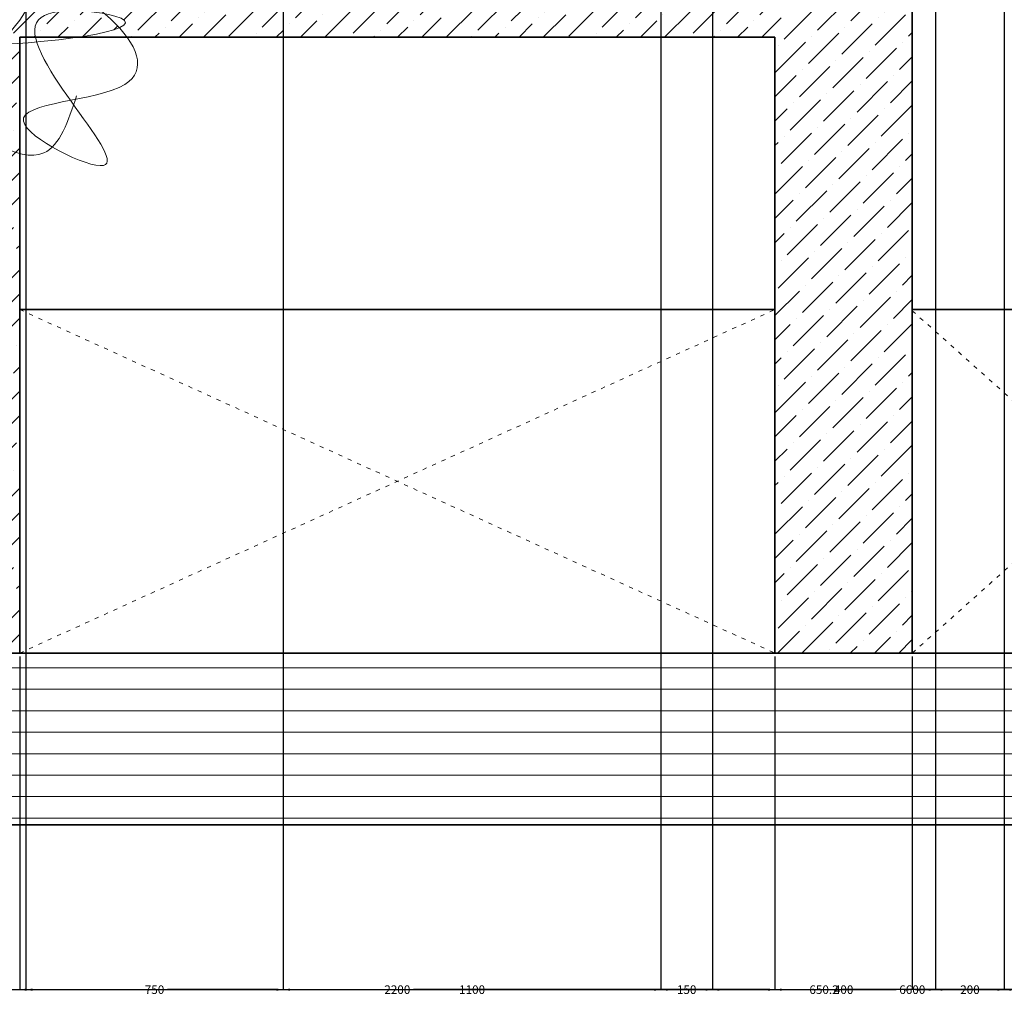
# Model space of a CAD drawing. Units: millimetres. Extents: x -692 to 9639, y -141 to 10345.
# Tile 3 of 19: x 3174 to 6042, y -141 to 2699. Entities that reach past the tile are written whole.
import ezdxf

# ---------------------------------------------------------------- set-up
doc = ezdxf.new("R2010")
doc.units = ezdxf.units.MM
doc.header["$MEASUREMENT"] = 0
doc.linetypes.add('ACAD_ISO03W100', pattern=[30, 12, -18])
for name, color, linetype, lineweight in [('A-ANNO-DIMS', 2, 'Continuous', 18), ('A-DOOR-SWNG', 3, 'ACAD_ISO03W100', 18), ('A-ELEV', 7, 'Continuous', 35), ('A-ELEV-PATT', 8, 'Continuous', 13), ('L-PLNT', 3, 'Continuous', 18)]:
    doc.layers.add(name, color=color, linetype=linetype, lineweight=lineweight)
doc.styles.get("Standard").update_dxf_attribs({"font": 'arial.ttf'})
doc.dimstyles.get("Standard").update_dxf_attribs({"dimtxt": 25, "dimasz": 20, "dimexe": 0.18, "dimexo": 10, "dimgap": 10, "dimtad": 0, "dimtih": 1, "dimtoh": 1, "dimdec": 0, "dimzin": 0, "dimdsep": 46, "dimtxsty": 'Standard', "dimcen": 10, "dimadec": 0, "dimazin": 0, "dimtfac": 1, "dimtdec": 0, "dimtofl": 0, "dimtmove": 0, "dimatfit": 3, "dimfxl": 1, "dimtolj": 1, "dimtzin": 0, "dimarcsym": 0})

# ---------------------------------------------------------------- blocks, each defined once
blk = doc.blocks.new('*D6')
at = {"layer": 'A-ANNO-DIMS', "color": 0, "lineweight": -2, "transparency": 16777216}
for p, q in [((2473.7, 345.6), (2473.7, -124.6)), ((9073.7, 345.6), (9073.7, -124.6)), ((2493.7, -124.4), (5726.4, -124.4)), ((9053.7, -124.4), (5821.1, -124.4))]:
    blk.add_line(p, q, dxfattribs=at)
at = {"layer": 'A-ANNO-DIMS', "color": 0, "lineweight": -3, "transparency": 16777216}
for points in [[(2493.7, -121.1), (2493.7, -127.8), (2473.7, -124.4)], [(9053.7, -121.1), (9053.7, -127.8), (9073.7, -124.4)]]:
    blk.add_solid(points, dxfattribs=at)
at = {"layer": 'Defpoints', "color": 0, "lineweight": -3, "transparency": 16777216}
for p in [(2473.7, 355.6), (9073.7, 355.6), (9073.7, -124.4)]:
    blk.add_point(p, dxfattribs=at)
at = {"layer": 'A-ANNO-DIMS', "color": 0, "transparency": 16777216, "insert": (5773.7, -124.4), "char_height": 25, "attachment_point": 5}
blk.add_mtext('\\A1;6600', dxfattribs=at)
blk = doc.blocks.new('*D7')
at = {"layer": 'A-ANNO-DIMS', "color": 0, "lineweight": -2, "transparency": 16777216}
for p, q in [((8481.5, 9848.8), (-649.1, 9848.8)), ((-648.9, 9828.8), (-648.9, 5124.9)), ((-648.9, 375.6), (-648.9, 5079.4)), ((2463.7, 355.6), (-649.1, 355.6))]:
    blk.add_line(p, q, dxfattribs=at)
at = {"layer": 'A-ANNO-DIMS', "color": 0, "lineweight": -3, "transparency": 16777216}
for points in [[(-652.2, 9828.8), (-645.6, 9828.8), (-648.9, 9848.8)], [(-652.2, 375.6), (-645.6, 375.6), (-648.9, 355.6)]]:
    blk.add_solid(points, dxfattribs=at)
at = {"layer": 'Defpoints', "color": 0, "lineweight": -3, "transparency": 16777216}
for p in [(-648.9, 9848.8), (8491.5, 9848.8), (2473.7, 355.6)]:
    blk.add_point(p, dxfattribs=at)
at = {"layer": 'A-ANNO-DIMS', "color": 0, "transparency": 16777216, "insert": (-648.9, 5102.2), "char_height": 25, "attachment_point": 5}
blk.add_mtext('\\A1;9493', dxfattribs=at)
blk = doc.blocks.new('*D20')
at = {"layer": 'A-ANNO-DIMS', "color": 0, "lineweight": -2, "transparency": 16777216}
for p, q in [((3173.7, 845.6), (3173.7, -124.6)), ((5373.7, 845.6), (5373.7, -124.6)), ((3193.7, -124.4), (4226.2, -124.4)), ((5353.7, -124.4), (4321.2, -124.4))]:
    blk.add_line(p, q, dxfattribs=at)
at = {"layer": 'A-ANNO-DIMS', "color": 0, "lineweight": -3, "transparency": 16777216}
for points in [[(3193.7, -121.1), (3193.7, -127.8), (3173.7, -124.4)], [(5353.7, -121.1), (5353.7, -127.8), (5373.7, -124.4)]]:
    blk.add_solid(points, dxfattribs=at)
at = {"layer": 'Defpoints', "color": 0, "lineweight": -3, "transparency": 16777216}
for p in [(3173.7, 855.6), (5373.7, 855.6), (5373.7, -124.4)]:
    blk.add_point(p, dxfattribs=at)
at = {"layer": 'A-ANNO-DIMS', "color": 0, "transparency": 16777216, "insert": (4273.7, -124.4), "char_height": 25, "attachment_point": 5}
blk.add_mtext('\\A1;2200', dxfattribs=at)
blk = doc.blocks.new('*D21')
at = {"layer": 'A-ANNO-DIMS', "color": 0, "lineweight": -2, "transparency": 16777216}
for p, q in [((5373.7, 845.6), (5373.7, -124.6)), ((5773.7, 845.6), (5773.7, -124.6)), ((5393.7, -124.4), (5535.7, -124.4)), ((5753.7, -124.4), (5611.8, -124.4))]:
    blk.add_line(p, q, dxfattribs=at)
at = {"layer": 'A-ANNO-DIMS', "color": 0, "lineweight": -3, "transparency": 16777216}
for points in [[(5393.7, -121.1), (5393.7, -127.8), (5373.7, -124.4)], [(5753.7, -121.1), (5753.7, -127.8), (5773.7, -124.4)]]:
    blk.add_solid(points, dxfattribs=at)
at = {"layer": 'Defpoints', "color": 0, "lineweight": -3, "transparency": 16777216}
for p in [(5373.7, 855.6), (5773.7, 855.6), (5773.7, -124.4)]:
    blk.add_point(p, dxfattribs=at)
at = {"layer": 'A-ANNO-DIMS', "color": 0, "transparency": 16777216, "insert": (5573.7, -124.4), "char_height": 25, "attachment_point": 5}
blk.add_mtext('\\A1;400', dxfattribs=at)
blk = doc.blocks.new('*D22')
at = {"layer": 'A-ANNO-DIMS', "color": 0, "lineweight": -2, "transparency": 16777216}
for p, q in [((5773.7, 845.6), (5773.7, -124.6)), ((6891.7, 845.6), (6891.7, -124.6)), ((5793.7, -124.4), (6286.6, -124.4)), ((6871.7, -124.4), (6378.9, -124.4))]:
    blk.add_line(p, q, dxfattribs=at)
at = {"layer": 'A-ANNO-DIMS', "color": 0, "lineweight": -3, "transparency": 16777216}
for points in [[(5793.7, -121.1), (5793.7, -127.8), (5773.7, -124.4)], [(6871.7, -121.1), (6871.7, -127.8), (6891.7, -124.4)]]:
    blk.add_solid(points, dxfattribs=at)
at = {"layer": 'Defpoints', "color": 0, "lineweight": -3, "transparency": 16777216}
for p in [(5773.7, 855.6), (6891.7, 855.6), (6891.7, -124.4)]:
    blk.add_point(p, dxfattribs=at)
at = {"layer": 'A-ANNO-DIMS', "color": 0, "transparency": 16777216, "insert": (6332.7, -124.4), "char_height": 25, "attachment_point": 5}
blk.add_mtext('\\A1;1118', dxfattribs=at)
blk = doc.blocks.new('*D37')
at = {"layer": 'A-ANNO-DIMS', "color": 0, "lineweight": -2, "transparency": 16777216}
for p, q in [((3941.5, 3412.8), (3941.5, -124.6)), ((3191.5, 2838.3), (3191.5, -124.6)), ((3211.5, -124.4), (3529.1, -124.4)), ((3921.5, -124.4), (3604, -124.4))]:
    blk.add_line(p, q, dxfattribs=at)
at = {"layer": 'A-ANNO-DIMS', "color": 0, "lineweight": -3, "transparency": 16777216}
for points in [[(3211.5, -121.1), (3211.5, -127.8), (3191.5, -124.4)], [(3921.5, -121.1), (3921.5, -127.8), (3941.5, -124.4)]]:
    blk.add_solid(points, dxfattribs=at)
at = {"layer": 'Defpoints', "color": 0, "lineweight": -3, "transparency": 16777216}
for p in [(3941.5, 3422.8), (3191.5, 2848.3), (3941.5, -124.4)]:
    blk.add_point(p, dxfattribs=at)
at = {"layer": 'A-ANNO-DIMS', "color": 0, "transparency": 16777216, "insert": (3566.5, -124.4), "char_height": 25, "attachment_point": 5}
blk.add_mtext('\\A1;750', dxfattribs=at)
blk = doc.blocks.new('*D38')
at = {"layer": 'A-ANNO-DIMS', "color": 0, "lineweight": -2, "transparency": 16777216}
for p, q in [((3941.5, 3412.8), (3941.5, -124.6)), ((5041.5, 3038.3), (5041.5, -124.6)), ((3961.5, -124.4), (4445.4, -124.4)), ((5021.5, -124.4), (4537.7, -124.4))]:
    blk.add_line(p, q, dxfattribs=at)
at = {"layer": 'A-ANNO-DIMS', "color": 0, "lineweight": -3, "transparency": 16777216}
for points in [[(3961.5, -121.1), (3961.5, -127.8), (3941.5, -124.4)], [(5021.5, -121.1), (5021.5, -127.8), (5041.5, -124.4)]]:
    blk.add_solid(points, dxfattribs=at)
at = {"layer": 'Defpoints', "color": 0, "lineweight": -3, "transparency": 16777216}
for p in [(3941.5, 3422.8), (5041.5, 3048.3), (5041.5, -124.4)]:
    blk.add_point(p, dxfattribs=at)
at = {"layer": 'A-ANNO-DIMS', "color": 0, "transparency": 16777216, "insert": (4491.5, -124.4), "char_height": 25, "attachment_point": 5}
blk.add_mtext('\\A1;1100', dxfattribs=at)
blk = doc.blocks.new('*D39')
at = {"layer": 'A-ANNO-DIMS', "color": 0, "lineweight": -2, "transparency": 16777216}
for p, q in [((5191.5, 3588.3), (5191.5, -124.6)), ((5041.5, 3038.3), (5041.5, -124.6)), ((5061.5, -124.4), (5080.1, -124.4)), ((5171.5, -124.4), (5152.9, -124.4))]:
    blk.add_line(p, q, dxfattribs=at)
at = {"layer": 'A-ANNO-DIMS', "color": 0, "lineweight": -3, "transparency": 16777216}
for points in [[(5061.5, -121.1), (5061.5, -127.8), (5041.5, -124.4)], [(5171.5, -121.1), (5171.5, -127.8), (5191.5, -124.4)]]:
    blk.add_solid(points, dxfattribs=at)
at = {"layer": 'Defpoints', "color": 0, "lineweight": -3, "transparency": 16777216}
for p in [(5191.5, 3598.3), (5041.5, 3048.3), (5191.5, -124.4)]:
    blk.add_point(p, dxfattribs=at)
at = {"layer": 'A-ANNO-DIMS', "color": 0, "transparency": 16777216, "insert": (5116.5, -124.4), "char_height": 25, "attachment_point": 5}
blk.add_mtext('\\A1;150', dxfattribs=at)
blk = doc.blocks.new('*D40')
at = {"layer": 'A-ANNO-DIMS', "color": 0, "lineweight": -2, "transparency": 16777216}
for p, q in [((5191.5, 3588.3), (5191.5, -124.6)), ((5841.7, 3588.3), (5841.7, -124.6)), ((5211.5, -124.4), (5464.5, -124.4)), ((5821.7, -124.4), (5568.8, -124.4))]:
    blk.add_line(p, q, dxfattribs=at)
at = {"layer": 'A-ANNO-DIMS', "color": 0, "lineweight": -3, "transparency": 16777216}
for points in [[(5211.5, -121.1), (5211.5, -127.8), (5191.5, -124.4)], [(5821.7, -121.1), (5821.7, -127.8), (5841.7, -124.4)]]:
    blk.add_solid(points, dxfattribs=at)
at = {"layer": 'Defpoints', "color": 0, "lineweight": -3, "transparency": 16777216}
for p in [(5191.5, 3598.3), (5841.7, 3598.3), (5841.7, -124.4)]:
    blk.add_point(p, dxfattribs=at)
at = {"layer": 'A-ANNO-DIMS', "color": 0, "transparency": 16777216, "insert": (5516.6, -124.4), "char_height": 25, "attachment_point": 5}
blk.add_mtext('\\A1;650.2', dxfattribs=at)
blk = doc.blocks.new('*D41')
at = {"layer": 'A-ANNO-DIMS', "color": 0, "lineweight": -2, "transparency": 16777216}
for p, q in [((5841.7, 3588.3), (5841.7, -124.6)), ((6041.7, 3588.3), (6041.7, -124.6)), ((5861.7, -124.4), (5904, -124.4)), ((6021.7, -124.4), (5979.5, -124.4))]:
    blk.add_line(p, q, dxfattribs=at)
at = {"layer": 'A-ANNO-DIMS', "color": 0, "lineweight": -3, "transparency": 16777216}
for points in [[(5861.7, -121.1), (5861.7, -127.8), (5841.7, -124.4)], [(6021.7, -121.1), (6021.7, -127.8), (6041.7, -124.4)]]:
    blk.add_solid(points, dxfattribs=at)
at = {"layer": 'Defpoints', "color": 0, "lineweight": -3, "transparency": 16777216}
for p in [(5841.7, 3598.3), (6041.7, 3598.3), (6041.7, -124.4)]:
    blk.add_point(p, dxfattribs=at)
at = {"layer": 'A-ANNO-DIMS', "color": 0, "transparency": 16777216, "insert": (5941.7, -124.4), "char_height": 25, "attachment_point": 5}
blk.add_mtext('\\A1;200', dxfattribs=at)
blk = doc.blocks.new('*D42')
at = {"layer": 'A-ANNO-DIMS', "color": 0, "lineweight": -2, "transparency": 16777216}
for p, q in [((6041.7, 3588.3), (6041.7, -124.6)), ((6691.7, 3588.3), (6691.7, -124.6)), ((6061.7, -124.4), (6329.1, -124.4)), ((6671.7, -124.4), (6404.4, -124.4))]:
    blk.add_line(p, q, dxfattribs=at)
at = {"layer": 'A-ANNO-DIMS', "color": 0, "lineweight": -3, "transparency": 16777216}
for points in [[(6061.7, -121.1), (6061.7, -127.8), (6041.7, -124.4)], [(6671.7, -121.1), (6671.7, -127.8), (6691.7, -124.4)]]:
    blk.add_solid(points, dxfattribs=at)
at = {"layer": 'Defpoints', "color": 0, "lineweight": -3, "transparency": 16777216}
for p in [(6041.7, 3598.3), (6691.7, 3598.3), (6691.7, -124.4)]:
    blk.add_point(p, dxfattribs=at)
at = {"layer": 'A-ANNO-DIMS', "color": 0, "transparency": 16777216, "insert": (6366.7, -124.4), "char_height": 25, "attachment_point": 5}
blk.add_mtext('\\A1;650', dxfattribs=at)

msp = doc.modelspace()

# ---------------------------------------------------------------- hatches: boundary and pattern name
at = {"layer": 'A-ELEV-PATT'}
h = msp.add_hatch(dxfattribs=at)
h.set_pattern_fill('ANSI36', color=256, scale=400)
edge = h.paths.add_edge_path()
edge.add_spline(control_points=[(3173.746, 2309.965), (3085.901, 2332.226), (2969.139, 2424.713), (2876.436, 2493.45)], knot_values=[20955.88576955, 20955.88576955, 20955.88576955, 20955.88576955, 21219.85539585, 21219.85539585, 21219.85539585, 21219.85539585], degree=3, periodic=0)
edge.add_spline(control_points=[(2876.436, 2493.45), (2855.134, 2468.311), (2819.135, 2451.154), (2773.746, 2440.514)], knot_values=[5238.08213467, 5238.08213467, 5238.08213467, 5238.08213467, 5382.8513026, 5382.8513026, 5382.8513026, 5382.8513026], degree=3, periodic=0)
edge.add_line((2773.746, 2440.514), (2773.746, 2354.397))
edge.add_spline(control_points=[(2773.746, 2354.397), (2777.278, 2343.918), (2780.812, 2333.449), (2784.279, 2323.093)], knot_values=[20514.20511429, 20514.20511429, 20514.20511429, 20514.20511429, 20537.39604293, 20537.39604293, 20537.39604293, 20537.39604293], degree=3, periodic=0)
edge.add_spline(control_points=[(2784.279, 2323.093), (2849.257, 2305.468), (3007.384, 2255.171), (2928.441, 2185.016), (2819.76, 2148.371)], knot_values=[1896.27813718, 1896.27813718, 1896.27813718, 1896.27813718, 2077.70067144, 2424.51760392, 2424.51760392, 2424.51760392, 2424.51760392], degree=3, periodic=0)
edge.add_spline(control_points=[(2819.76, 2148.371), (2817.899, 2146.748), (2815.52, 2145.926), (2812.57, 2145.987)], knot_values=[20304.87329269, 20304.87329269, 20304.87329269, 20304.87329269, 20326.21847821, 20326.21847821, 20326.21847821, 20326.21847821], degree=3, periodic=0)
edge.add_spline(control_points=[(2812.57, 2145.987), (2800.291, 2141.985), (2787.329, 2138.102), (2773.746, 2134.363)], knot_values=[1850.39591646, 1850.39591646, 1850.39591646, 1850.39591646, 1888.716341, 1888.716341, 1888.716341, 1888.716341], degree=3, periodic=0)
edge.add_line((2773.746, 2134.363), (2773.746, 855.575))
edge.add_line((2773.746, 855.575), (3173.746, 855.575))
edge.add_line((3173.746, 855.575), (3173.746, 2309.965))
edge = h.paths.add_edge_path()
edge.add_spline(control_points=[(3420.651, 2717.101), (3368.378, 2761.363), (3299.425, 2803.396), (3225.3, 2834.508)], knot_values=[12552.99587302, 12552.99587302, 12552.99587302, 12552.99587302, 12712.02358035, 12712.02358035, 12712.02358035, 12712.02358035], degree=3, periodic=0)
edge.add_spline(control_points=[(3225.3, 2834.508), (3218.267, 2754.576), (3174.644, 2682.922), (3107.112, 2626.403)], knot_values=[8572.46293399, 8572.46293399, 8572.46293399, 8572.46293399, 8814.86919927, 8814.86919927, 8814.86919927, 8814.86919927], degree=3, periodic=0)
edge.add_spline(control_points=[(3107.112, 2626.403), (3129.755, 2627.593), (3152.034, 2628.996), (3173.746, 2630.586)], knot_values=[10558.19039557, 10558.19039557, 10558.19039557, 10558.19039557, 10599.03834951, 10599.03834951, 10599.03834951, 10599.03834951], degree=3, periodic=0)
edge.add_line((3173.746, 2630.586), (3173.746, 2648.27))
edge.add_line((3173.746, 2648.27), (3219.774, 2648.27))
edge.add_spline(control_points=[(3219.774, 2648.27), (3215.509, 2669.279), (3223.352, 2735.229), (3357.845, 2728.872), (3420.651, 2717.101)], knot_values=[11042.13010686, 11042.13010686, 11042.13010686, 11042.13010686, 11110.4948836, 11298.41454305, 11298.41454305, 11298.41454305, 11298.41454305], degree=3, periodic=0)
edge = h.paths.add_edge_path()
edge.add_spline(control_points=[(3107.112, 2626.403), (3174.644, 2682.922), (3218.267, 2754.576), (3225.3, 2834.508)], knot_values=[8572.46293399, 8572.46293399, 8572.46293399, 8572.46293399, 8814.86919927, 8814.86919927, 8814.86919927, 8814.86919927], degree=3, periodic=0)
edge.add_spline(control_points=[(3225.3, 2834.508), (3213.709, 2839.374), (3201.991, 2843.972), (3190.19, 2848.27)], knot_values=[12712.02358035, 12712.02358035, 12712.02358035, 12712.02358035, 12736.8923557, 12736.8923557, 12736.8923557, 12736.8923557], degree=3, periodic=0)
edge.add_line((3190.19, 2848.27), (2928.387, 2848.27))
edge.add_spline(control_points=[(2928.387, 2848.27), (2886.081, 2816.098), (2840.884, 2784.767), (2798.089, 2758.256)], knot_values=[14939.29716066, 14939.29716066, 14939.29716066, 14939.29716066, 15046.25935392, 15046.25935392, 15046.25935392, 15046.25935392], degree=3, periodic=0)
edge.add_spline(control_points=[(2798.089, 2758.256), (2836.427, 2711.897), (2866.292, 2664.879), (2883.022, 2622.327)], knot_values=[5561.23366662, 5561.23366662, 5561.23366662, 5561.23366662, 5704.57044689, 5704.57044689, 5704.57044689, 5704.57044689], degree=3, periodic=0)
edge.add_spline(control_points=[(2883.022, 2622.327), (2956.927, 2620.92), (3033.919, 2622.554), (3107.112, 2626.403)], knot_values=[10426.14846168, 10426.14846168, 10426.14846168, 10426.14846168, 10558.19039557, 10558.19039557, 10558.19039557, 10558.19039557], degree=3, periodic=0)
edge = h.paths.add_edge_path()
edge.add_spline(control_points=[(3173.746, 2630.586), (3152.034, 2628.996), (3129.755, 2627.593), (3107.112, 2626.403)], knot_values=[10558.19039557, 10558.19039557, 10558.19039557, 10558.19039557, 10599.03834951, 10599.03834951, 10599.03834951, 10599.03834951], degree=3, periodic=0)
edge.add_spline(control_points=[(3107.112, 2626.403), (3049.969, 2578.578), (2975.708, 2541.59), (2892.012, 2519.592)], knot_values=[8367.34849038, 8367.34849038, 8367.34849038, 8367.34849038, 8572.46293399, 8572.46293399, 8572.46293399, 8572.46293399], degree=3, periodic=0)
edge.add_spline(control_points=[(2892.012, 2519.592), (2888.384, 2510.058), (2883.137, 2501.359), (2876.436, 2493.45)], knot_values=[5382.8513026, 5382.8513026, 5382.8513026, 5382.8513026, 5428.39625745, 5428.39625745, 5428.39625745, 5428.39625745], degree=3, periodic=0)
edge.add_spline(control_points=[(2876.436, 2493.45), (2969.139, 2424.713), (3085.901, 2332.226), (3173.746, 2309.965)], knot_values=[20955.88576955, 20955.88576955, 20955.88576955, 20955.88576955, 21219.85539585, 21219.85539585, 21219.85539585, 21219.85539585], degree=3, periodic=0)
edge.add_line((3173.746, 2309.965), (3173.746, 2630.586))
edge = h.paths.add_edge_path(flags=17)
edge.add_spline(control_points=[(2819.76, 2148.371), (2928.441, 2185.016), (3007.384, 2255.171), (2849.257, 2305.468), (2784.279, 2323.093)], knot_values=[1896.27813718, 1896.27813718, 1896.27813718, 1896.27813718, 2243.09506965, 2424.51760392, 2424.51760392, 2424.51760392, 2424.51760392], degree=3, periodic=0)
edge.add_spline(control_points=[(2784.279, 2323.093), (2812.387, 2239.151), (2836.152, 2162.664), (2819.76, 2148.371)], knot_values=[20326.21847821, 20326.21847821, 20326.21847821, 20326.21847821, 20514.20511429, 20514.20511429, 20514.20511429, 20514.20511429], degree=3, periodic=0)
edge = h.paths.add_edge_path(flags=17)
edge.add_spline(control_points=[(2819.76, 2148.371), (2836.152, 2162.664), (2812.387, 2239.151), (2784.279, 2323.093)], knot_values=[20326.21847821, 20326.21847821, 20326.21847821, 20326.21847821, 20514.20511429, 20514.20511429, 20514.20511429, 20514.20511429], degree=3, periodic=0)
edge.add_spline(control_points=[(2784.279, 2323.093), (2780.798, 2324.038), (2777.286, 2324.983), (2773.746, 2325.93)], knot_values=[2424.51760392, 2424.51760392, 2424.51760392, 2424.51760392, 2434.23800618, 2434.23800618, 2434.23800618, 2434.23800618], degree=3, periodic=0)
edge.add_line((2773.746, 2325.93), (2773.746, 2166.486))
edge.add_spline(control_points=[(2773.746, 2166.486), (2790.303, 2153.967), (2803.9, 2146.166), (2812.57, 2145.987)], knot_values=[20242.12265912, 20242.12265912, 20242.12265912, 20242.12265912, 20304.87329269, 20304.87329269, 20304.87329269, 20304.87329269], degree=3, periodic=0)
edge.add_spline(control_points=[(2812.57, 2145.987), (2814.994, 2146.777), (2817.39, 2147.572), (2819.76, 2148.371)], knot_values=[1888.716341, 1888.716341, 1888.716341, 1888.716341, 1896.27813718, 1896.27813718, 1896.27813718, 1896.27813718], degree=3, periodic=0)
edge = h.paths.add_edge_path()
edge.add_spline(control_points=[(2892.012, 2519.592), (2893.653, 2523.907), (2902.094, 2552.818), (2896.12, 2589.012), (2883.022, 2622.327)], knot_values=[5428.39625745, 5428.39625745, 5428.39625745, 5428.39625745, 5449.01011401, 5561.23366662, 5561.23366662, 5561.23366662, 5561.23366662], degree=3, periodic=0)
edge.add_spline(control_points=[(2883.022, 2622.327), (2845.501, 2623.042), (2808.775, 2624.54), (2773.746, 2626.93)], knot_values=[10359.11175247, 10359.11175247, 10359.11175247, 10359.11175247, 10426.14846168, 10426.14846168, 10426.14846168, 10426.14846168], degree=3, periodic=0)
edge.add_line((2773.746, 2626.93), (2773.746, 2561.8))
edge.add_spline(control_points=[(2773.746, 2561.8), (2795.257, 2551.206), (2822.448, 2532.82), (2853.096, 2510.59)], knot_values=[20841.44589883, 20841.44589883, 20841.44589883, 20841.44589883, 20933.19502211, 20933.19502211, 20933.19502211, 20933.19502211], degree=3, periodic=0)
edge.add_spline(control_points=[(2853.096, 2510.59), (2866.269, 2513.232), (2879.25, 2516.238), (2892.012, 2519.592)], knot_values=[8336.07392909, 8336.07392909, 8336.07392909, 8336.07392909, 8367.34849038, 8367.34849038, 8367.34849038, 8367.34849038], degree=3, periodic=0)
edge = h.paths.add_edge_path(flags=17)
edge.add_spline(control_points=[(2892.012, 2519.592), (2975.708, 2541.59), (3049.969, 2578.578), (3107.112, 2626.403)], knot_values=[8367.34849038, 8367.34849038, 8367.34849038, 8367.34849038, 8572.46293399, 8572.46293399, 8572.46293399, 8572.46293399], degree=3, periodic=0)
edge.add_spline(control_points=[(3107.112, 2626.403), (3033.919, 2622.554), (2956.927, 2620.92), (2883.022, 2622.327)], knot_values=[10426.14846168, 10426.14846168, 10426.14846168, 10426.14846168, 10558.19039557, 10558.19039557, 10558.19039557, 10558.19039557], degree=3, periodic=0)
edge.add_spline(control_points=[(2883.022, 2622.327), (2896.12, 2589.012), (2902.094, 2552.818), (2893.653, 2523.907), (2892.012, 2519.592)], knot_values=[5428.39625745, 5428.39625745, 5428.39625745, 5428.39625745, 5540.61981006, 5561.23366662, 5561.23366662, 5561.23366662, 5561.23366662], degree=3, periodic=0)
edge = h.paths.add_edge_path()
edge.add_spline(control_points=[(2773.746, 2440.514), (2819.135, 2451.154), (2855.134, 2468.311), (2876.436, 2493.45)], knot_values=[5238.08213467, 5238.08213467, 5238.08213467, 5238.08213467, 5382.8513026, 5382.8513026, 5382.8513026, 5382.8513026], degree=3, periodic=0)
edge.add_spline(control_points=[(2876.436, 2493.45), (2868.467, 2499.359), (2860.676, 2505.092), (2853.096, 2510.59)], knot_values=[20933.19502211, 20933.19502211, 20933.19502211, 20933.19502211, 20955.88576955, 20955.88576955, 20955.88576955, 20955.88576955], degree=3, periodic=0)
edge.add_spline(control_points=[(2853.096, 2510.59), (2827.314, 2505.418), (2800.796, 2501.637), (2773.746, 2499.359)], knot_values=[8274.86392127, 8274.86392127, 8274.86392127, 8274.86392127, 8336.07392909, 8336.07392909, 8336.07392909, 8336.07392909], degree=3, periodic=0)
edge.add_line((2773.746, 2499.359), (2773.746, 2440.514))
edge = h.paths.add_edge_path()
edge.add_spline(control_points=[(2883.022, 2622.327), (2866.292, 2664.879), (2836.427, 2711.897), (2798.089, 2758.256)], knot_values=[5561.23366662, 5561.23366662, 5561.23366662, 5561.23366662, 5704.57044689, 5704.57044689, 5704.57044689, 5704.57044689], degree=3, periodic=0)
edge.add_spline(control_points=[(2798.089, 2758.256), (2789.874, 2753.166), (2781.747, 2748.254), (2773.746, 2743.548)], knot_values=[15046.25935392, 15046.25935392, 15046.25935392, 15046.25935392, 15066.79294618, 15066.79294618, 15066.79294618, 15066.79294618], degree=3, periodic=0)
edge.add_line((2773.746, 2743.548), (2773.746, 2626.93))
edge.add_spline(control_points=[(2773.746, 2626.93), (2808.775, 2624.54), (2845.501, 2623.042), (2883.022, 2622.327)], knot_values=[10359.11175247, 10359.11175247, 10359.11175247, 10359.11175247, 10426.14846168, 10426.14846168, 10426.14846168, 10426.14846168], degree=3, periodic=0)
edge = h.paths.add_edge_path()
edge.add_spline(control_points=[(2798.089, 2758.256), (2840.884, 2784.767), (2886.081, 2816.098), (2928.387, 2848.27)], knot_values=[14939.29716066, 14939.29716066, 14939.29716066, 14939.29716066, 15046.25935392, 15046.25935392, 15046.25935392, 15046.25935392], degree=3, periodic=0)
edge.add_line((2928.387, 2848.27), (2773.746, 2848.27))
edge.add_line((2773.746, 2848.27), (2773.746, 2786.349))
edge.add_spline(control_points=[(2773.746, 2786.349), (2782.183, 2777.04), (2790.311, 2767.662), (2798.089, 2758.256)], knot_values=[5704.57044689, 5704.57044689, 5704.57044689, 5704.57044689, 5733.65273084, 5733.65273084, 5733.65273084, 5733.65273084], degree=3, periodic=0)
edge = h.paths.add_edge_path()
edge.add_spline(control_points=[(3463.702, 2676.006), (3451.141, 2689.747), (3436.681, 2703.529), (3420.651, 2717.101)], knot_values=[12504.23047843, 12504.23047843, 12504.23047843, 12504.23047843, 12552.99587302, 12552.99587302, 12552.99587302, 12552.99587302], degree=3, periodic=0)
edge.add_spline(control_points=[(3420.651, 2717.101), (3357.845, 2728.872), (3223.352, 2735.229), (3215.509, 2669.279), (3219.774, 2648.27)], knot_values=[11042.13010686, 11042.13010686, 11042.13010686, 11042.13010686, 11230.04976631, 11298.41454305, 11298.41454305, 11298.41454305, 11298.41454305], degree=3, periodic=0)
edge.add_line((3219.774, 2648.27), (3341.426, 2648.27))
edge.add_spline(control_points=[(3341.426, 2648.27), (3397.595, 2656.506), (3440.895, 2666.057), (3463.702, 2676.006)], knot_values=[10715.9300286, 10715.9300286, 10715.9300286, 10715.9300286, 10852.53626518, 10852.53626518, 10852.53626518, 10852.53626518], degree=3, periodic=0)
edge = h.paths.add_edge_path()
edge.add_spline(control_points=[(2853.096, 2510.59), (2822.448, 2532.82), (2795.257, 2551.206), (2773.746, 2561.8)], knot_values=[20841.44589883, 20841.44589883, 20841.44589883, 20841.44589883, 20933.19502211, 20933.19502211, 20933.19502211, 20933.19502211], degree=3, periodic=0)
edge.add_line((2773.746, 2561.8), (2773.746, 2499.359))
edge.add_spline(control_points=[(2773.746, 2499.359), (2800.796, 2501.637), (2827.314, 2505.418), (2853.096, 2510.59)], knot_values=[8274.86392127, 8274.86392127, 8274.86392127, 8274.86392127, 8336.07392909, 8336.07392909, 8336.07392909, 8336.07392909], degree=3, periodic=0)
h = msp.add_hatch(dxfattribs=at)
h.set_pattern_fill('ANSI36', color=256, scale=400)
edge = h.paths.add_edge_path()
edge.add_line((5773.746, 2848.27), (3226.144, 2848.27))
edge.add_spline(control_points=[(3226.144, 2848.27), (3225.984, 2843.657), (3225.702, 2839.069), (3225.3, 2834.508)], knot_values=[8814.86919927, 8814.86919927, 8814.86919927, 8814.86919927, 8828.69997321, 8828.69997321, 8828.69997321, 8828.69997321], degree=3, periodic=0)
edge.add_spline(control_points=[(3225.3, 2834.508), (3299.425, 2803.396), (3368.378, 2761.363), (3420.651, 2717.101)], knot_values=[12552.99587302, 12552.99587302, 12552.99587302, 12552.99587302, 12712.02358035, 12712.02358035, 12712.02358035, 12712.02358035], degree=3, periodic=0)
edge.add_spline(control_points=[(3420.651, 2717.101), (3432.322, 2714.914), (3488.975, 2701.706), (3489.525, 2687.271), (3463.702, 2676.006)], knot_values=[10852.53626518, 10852.53626518, 10852.53626518, 10852.53626518, 10887.45464539, 11042.13010686, 11042.13010686, 11042.13010686, 11042.13010686], degree=3, periodic=0)
edge.add_spline(control_points=[(3463.702, 2676.006), (3472.194, 2666.716), (3479.817, 2657.445), (3486.469, 2648.27)], knot_values=[12471.26094935, 12471.26094935, 12471.26094935, 12471.26094935, 12504.23047843, 12504.23047843, 12504.23047843, 12504.23047843], degree=3, periodic=0)
edge.add_line((3486.469, 2648.27), (5373.746, 2648.27))
edge.add_line((5373.746, 2648.27), (5373.746, 855.575))
edge.add_line((5373.746, 855.575), (5773.746, 855.575))
edge.add_line((5773.746, 855.575), (5773.746, 2848.27))
h = msp.add_hatch(dxfattribs=at)
h.set_pattern_fill('LINE', color=256, scale=500)
h.paths.add_polyline_path([(9073.746, 855.575), (8773.746, 855.575), (7273.746, 855.575), (2773.746, 855.575), (2473.746, 855.575), (2473.746, 355.575), (9073.746, 355.575)])

# ---------------------------------------------------------------- linework, layer by layer
at = {"layer": 'A-DOOR-SWNG'}
for p, q in [((3173.746, 855.575), (5373.746, 1855.575)), ((3173.746, 1855.575), (5373.746, 855.575)), ((5773.746, 855.575), (6891.746, 1855.575)), ((5773.746, 1851.922), (6891.746, 855.575))]:
    msp.add_line(p, q, dxfattribs=at)
at = {"layer": 'A-ELEV'}
for p, q in [((5773.746, 2848.27), (5773.746, 855.575)), ((3173.746, 2648.27), (3173.746, 855.575)), ((3173.746, 2648.27), (5373.746, 2648.27)), ((5373.746, 2648.27), (5373.746, 855.575)), ((5373.746, 1855.575), (3173.746, 1855.575)), ((6891.746, 1855.575), (5773.746, 1855.575)), ((7273.746, 855.575), (2773.746, 855.575)), ((2473.746, 355.575), (9073.746, 355.575))]:
    msp.add_line(p, q, dxfattribs=at)
at = {"layer": 'L-PLNT'}
msp.add_open_spline([(2323.333, 2214.265), (2305.649, 2163.243), (2257.888, 2025.445), (1935.117, 1924.822), (1413.715, 2416.586), (2206.705, 1935.154), (3264.488, 2224.597), (2555.092, 2370.602), (2159.771, 2527.783), (2008.053, 1993.707), (1823.12, 2332.645), (1174.123, 2625.596), (1944.245, 2620.173), (2297.612, 2431.636), (3340.282, 2329.714), (2122.894, 3461.216), (2087.569, 2088.062), (1584.671, 3289.033), (2501.939, 2207.058), (3524.445, 2766.924), (2798.31, 3455.317), (2706.153, 2954.832), (2166.187, 2516.526), (3968.598, 2664.724), (2990, 2769.255), (3688.565, 2108.449), (2982.144, 2461.359), (3771.592, 2459.928), (3182.433, 2965.822), (2527.115, 2819.368), (3221.379, 3433.367), (3370.439, 2797.07), (2591.814, 2891.377), (3329.128, 3168.682), (2633.805, 2580.308), (2320.472, 2701.322), (1352.991, 2495.29), (1929.878, 2444.347), (2406.24, 1895.881), (1637.78, 2788.225), (1673.077, 2130.341), (1834.638, 1713.755), (2155.278, 2063.673), (2496.635, 2611.137), (2362.564, 2025.688), (2789.19, 1894.041), (2353.111, 2630.053), (3000.854, 1872.269), (2485.666, 2949.85), (3219.61, 2114.193), (3315.543, 2405.105), (3339.585, 2478.009)], degree=3, knots=[0, 0, 0, 0, 156.01346293, 421.35741543, 891.47725045, 1326.49022079, 2243.09506965, 2561.11240616, 3034.23136561, 3344.76171519, 3437.70824639, 4024.35592839, 4525.63722229, 4755.92435047, 5449.01011401, 6226.81953685, 6823.80489855, 7287.95261826, 8086.77706947, 8892.28439463, 9398.99039818, 9802.71434696, 10041.58770662, 11007.21172666, 11230.04976631, 11694.3239388, 11960.50265147, 12274.78503374, 12794.79981033, 13145.39931196, 13672.14990348, 13935.42377748, 14348.98904743, 14621.34829061, 15077.00752658, 15638.15277437, 16264.82873645, 16548.19934354, 16952.30560132, 17525.13857657, 17920.46774586, 18221.89473837, 18637.38469135, 19024.43489898, 19426.39819861, 19566.65499761, 19968.27543453, 20304.87329269, 20724.59660574, 21299.21696159, 21491.37708517, 21491.37708517, 21491.37708517, 21491.37708517], dxfattribs=at)

# ---------------------------------------------------------------- dimensions: what is measured, and where the dimension line sits
at = {"layer": 'A-ANNO-DIMS'}
dim = msp.add_linear_dim(base=(-648.912, 9848.772), p1=(2473.746, 355.575), p2=(8491.547, 9848.772), angle=90, dimstyle='Standard', override={"dimdec": 0, "dimlfac": 1, "dimrnd": 0, "dimzin": 0, "dimdsep": 46, "dimlunit": 2}, dxfattribs=at)
dim.commit()
dim.dimension.update_dxf_attribs({"geometry": '*D7', "text_midpoint": (-648.912, 5102.173)})
for base, p1, p2, override, picture, middle in [((5191.547, -124.425), (5041.547, 3048.27), (5191.547, 3598.27), {"dimdec": 0, "dimlfac": 1, "dimrnd": 0, "dimzin": 0, "dimdsep": 46, "dimlunit": 2}, '*D39', (5116.547, -124.425)), ((5841.746, -124.425), (5191.547, 3598.27), (5841.746, 3598.27), {"dimdec": 1, "dimlfac": 1, "dimrnd": 0, "dimzin": 0, "dimdsep": 46, "dimlunit": 2}, '*D40', (5516.646, -124.425)), ((6041.746, -124.425), (5841.746, 3598.27), (6041.746, 3598.27), {"dimdec": 0, "dimlfac": 1, "dimrnd": 0, "dimzin": 0, "dimdsep": 46, "dimlunit": 2}, '*D41', (5941.746, -124.425)), ((6691.746, -124.425), (6041.746, 3598.27), (6691.746, 3598.27), {"dimdec": 0, "dimlfac": 1, "dimrnd": 0, "dimzin": 0, "dimdsep": 46, "dimlunit": 2}, '*D42', (6366.746, -124.425)), ((3941.547, -124.425), (3191.547, 2848.27), (3941.547, 3422.772), {"dimdec": 0, "dimlfac": 1, "dimrnd": 0, "dimzin": 0, "dimdsep": 46, "dimlunit": 2}, '*D37', (3566.547, -124.425)), ((5041.547, -124.425), (3941.547, 3422.772), (5041.547, 3048.27), {"dimdec": 0, "dimlfac": 1, "dimrnd": 0, "dimzin": 0, "dimdsep": 46, "dimlunit": 2}, '*D38', (4491.547, -124.425)), ((5373.746, -124.425), (3173.746, 855.575), (5373.746, 855.575), {"dimdec": 0, "dimlfac": 1, "dimrnd": 0, "dimzin": 0, "dimdsep": 46, "dimlunit": 2}, '*D20', (4273.746, -124.425)), ((5773.746, -124.425), (5373.746, 855.575), (5773.746, 855.575), {"dimdec": 0, "dimlfac": 1, "dimrnd": 0, "dimzin": 0, "dimdsep": 46, "dimlunit": 2}, '*D21', (5573.746, -124.425)), ((6891.746, -124.425), (5773.746, 855.575), (6891.746, 855.575), {"dimdec": 0, "dimlfac": 1, "dimrnd": 0, "dimzin": 0, "dimdsep": 46, "dimlunit": 2}, '*D22', (6332.746, -124.425)), ((9073.746, -124.425), (2473.746, 355.575), (9073.746, 355.575), {"dimdec": 0, "dimlfac": 1, "dimrnd": 0, "dimzin": 0, "dimdsep": 46, "dimlunit": 2}, '*D6', (5773.746, -124.425))]:
    dim = msp.add_linear_dim(base=base, p1=p1, p2=p2, dimstyle='Standard', override=override, dxfattribs=at)
    dim.commit()
    dim.dimension.update_dxf_attribs({"geometry": picture, "text_midpoint": middle})

doc.saveas('drawing.dxf')
